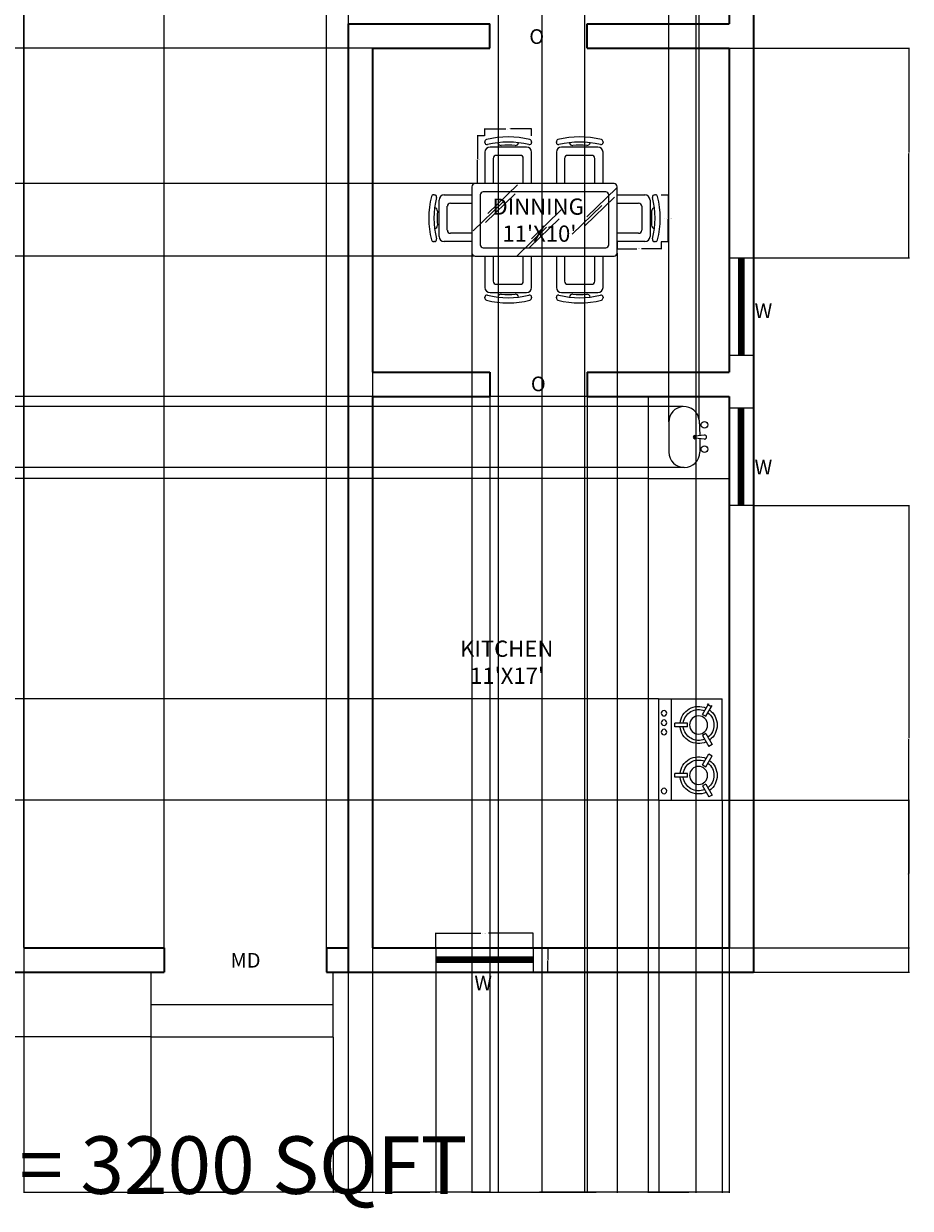
# Model space of a CAD drawing. Units: inches. Extents: x 318 to 927, y -1130 to 13.
# Tile 7 of 17: x 599 to 927, y -1130 to -692. Entities that reach past the tile are written whole.
import ezdxf

# ---------------------------------------------------------------- set-up
doc = ezdxf.new("R2010")
doc.units = ezdxf.units.IN
doc.header["$MEASUREMENT"] = 0
for name, color, linetype, lineweight in [('A-ANNO-DIMS', 1, 'Continuous', 18), ('A-ANNO-IDEN', 1, 'Continuous', 13), ('A-ANNO-TEXT', 8, 'Continuous', 25), ('A-AREA-IDEN', 8, 'Continuous', 18), ('A-EQPM', 50, 'Continuous', 18), ('A-FLOR-CASE', 50, 'Continuous', 18), ('A-FLOR-FIXT', 7, 'Continuous', 18), ('A-FLOR-STRS', 1, 'Continuous', 18), ('A-GLAZ-PATT', 5, 'Continuous', 9), ('wall', 1, 'Continuous', 35), ('win', 5, 'Continuous', 18)]:
    doc.layers.add(name, color=color, linetype=linetype, lineweight=lineweight)
doc.layers.add('furniture', color=50, linetype='Continuous', lineweight=13, transparency=0.8)
doc.styles.get("Standard").update_dxf_attribs({"font": 'arial.ttf'})
doc.dimstyles.get("Standard").update_dxf_attribs({"dimtxt": 0.18, "dimasz": 0.18, "dimexe": 0.18, "dimexo": 0.0625, "dimgap": 0.09, "dimtad": 0, "dimtih": 1, "dimtoh": 1, "dimdec": 1, "dimzin": 0, "dimdsep": 46, "dimlunit": 4, "dimtxsty": 'Standard', "dimcen": 0.09, "dimadec": 0, "dimazin": 0, "dimtfac": 1, "dimtdec": 1, "dimtofl": 0, "dimtmove": 0, "dimatfit": 3, "dimfxl": 1, "dimtolj": 1, "dimtzin": 0, "dimarcsym": 0})

# ---------------------------------------------------------------- blocks, each defined once
blk = doc.blocks.new('WIN-36IN')
for p, q in [((0, 36), (9, 36)), ((3.5, 36), (3.5, 0)), ((5.5, 36), (5.5, 0)), ((0, 0), (9, 0))]:
    blk.add_line(p, q)
blk = doc.blocks.new('CHAIR-DINING-SIDE')
for p, q in [((15.35, 13.5), (1.92, 13.5)), ((4.8, 15.13), (4.8, 15.25)), ((12.47, 15.13), (12.47, 15.25)), ((0, 11.76), (0, 11.36)), ((0, 11.58), (0, 0)), ((3.07, 9.28), (3.07, 0)), ((13.05, 10.43), (4.22, 10.43)), ((14.2, 0), (14.2, 9.28)), ((17.27, 11.36), (17.27, 11.76)), ((17.27, 0), (17.27, 11.58))]:
    blk.add_line(p, q)
for centre, radius, start, end in [((0.77, 15.54), 0.768, 104.147, 185.9216), ((-1.14, 15.34), 1.15, 354.0784, 5.9216), ((0.77, 15.15), 0.768, 174.0784, 284.3214), ((1.92, 11.58), 1.92, 90, 180), ((8.63, -15.67), 32.96, 75.853, 104.147), ((8.63, -15.67), 31.04, 75.6786, 104.3214), ((5.95, 15.25), 1.15, 186.0281, 274.9654), ((8.63, -15.67), 29.89, 85.0346, 94.9654), ((11.32, 15.25), 1.15, 265.0346, 353.9719), ((15.35, 11.58), 1.92, 0, 90), ((16.5, 15.15), 0.768, 255.6786, 5.9216), ((16.5, 15.54), 0.768, 354.0784, 75.853), ((18.41, 15.34), 1.15, 174.0784, 185.9216), ((4.22, 9.28), 1.15, 90, 180), ((13.05, 9.28), 1.15, 0, 90)]:
    blk.add_arc(centre, radius, start, end)
blk = doc.blocks.new('CHAIR-DINING-END')
for p, q in [((3.78, 1.92), (3.78, 15.35)), ((5.53, 17.27), (5.92, 17.27)), ((5.7, 17.27), (15.95, 17.27)), ((8.01, 14.2), (15.95, 14.2)), ((2.16, 12.47), (2.04, 12.47)), ((6.85, 4.22), (6.85, 13.05)), ((2.16, 4.8), (2.04, 4.8)), ((5.92, 0), (5.53, 0)), ((15.95, 0), (5.7, 0)), ((15.95, 3.07), (8.01, 3.07))]:
    blk.add_line(p, q)
for centre, radius, start, end in [((32.95, 8.63), 32.96, 165.853, 194.147), ((1.74, 16.5), 0.768, 84.0784, 165.853), ((1.94, 18.41), 1.15, 264.0784, 275.9216), ((32.95, 8.63), 31.04, 165.6786, 194.3214), ((2.14, 16.5), 0.768, 345.6786, 95.9216), ((5.7, 15.35), 1.92, 90, 180), ((8.01, 13.05), 1.15, 90, 180), ((2.04, 11.32), 1.15, 355.0346, 83.9719), ((32.95, 8.63), 29.89, 175.0346, 184.9654), ((2.04, 5.95), 1.15, 276.0281, 4.9654), ((1.74, 0.77), 0.768, 194.147, 275.9216), ((1.94, -1.14), 1.15, 84.0784, 95.9216), ((2.14, 0.77), 0.768, 264.0784, 14.3214), ((5.7, 1.92), 1.92, 180, 270), ((8.01, 4.22), 1.15, 180, 270)]:
    blk.add_arc(centre, radius, start, end)
blk = doc.blocks.new('*D11')
at = {"layer": 'A-ANNO-DIMS', "color": 0, "lineweight": -2, "transparency": 16777216}
for p, q in [((751.43, -1033.85), (751.43, -1028.33)), ((751.61, -1028.51), (768.05, -1028.51)), ((787.25, -1028.51), (770.81, -1028.51)), ((787.43, -1033.85), (787.43, -1028.33))]:
    blk.add_line(p, q, dxfattribs=at)
at = {"layer": 'A-ANNO-DIMS', "color": 0, "transparency": 16777216}
for points in [[(751.61, -1028.48), (751.61, -1028.54), (751.43, -1028.51)], [(787.25, -1028.48), (787.25, -1028.54), (787.43, -1028.51)]]:
    blk.add_solid(points, dxfattribs=at)
at = {"layer": 'Defpoints', "color": 0, "transparency": 16777216}
for p in [(787.43, -1028.51), (751.43, -1033.91), (787.43, -1033.91)]:
    blk.add_point(p, dxfattribs=at)
at = {"layer": 'A-ANNO-DIMS', "color": 0, "transparency": 16777216, "insert": (769.43, -1028.51), "char_height": 0.18, "attachment_point": 5}
blk.add_mtext('\\A1;WINDOW W 3\'-0" TYP.', dxfattribs=at)
blk = doc.blocks.new('*D12')
at = {"layer": 'A-ANNO-DIMS', "color": 0, "lineweight": -2, "transparency": 16777216}
for p, q in [((787.49, -1033.91), (793.01, -1033.91)), ((792.83, -1034.09), (792.83, -1038.23)), ((792.83, -1042.73), (792.83, -1038.59)), ((787.49, -1042.91), (793.01, -1042.91))]:
    blk.add_line(p, q, dxfattribs=at)
at = {"layer": 'A-ANNO-DIMS', "color": 0, "transparency": 16777216}
for points in [[(792.8, -1034.09), (792.86, -1034.09), (792.83, -1033.91)], [(792.8, -1042.73), (792.86, -1042.73), (792.83, -1042.91)]]:
    blk.add_solid(points, dxfattribs=at)
at = {"layer": 'Defpoints', "color": 0, "transparency": 16777216}
for p in [(787.43, -1033.91), (787.43, -1042.91), (792.83, -1042.91)]:
    blk.add_point(p, dxfattribs=at)
at = {"layer": 'A-ANNO-DIMS', "color": 0, "transparency": 16777216, "insert": (792.83, -1038.41), "char_height": 0.18, "attachment_point": 5}
blk.add_mtext('\\A1;0\'-9" TYP.', dxfattribs=at)
blk = doc.blocks.new('*D15')
at = {"layer": 'A-ANNO-DIMS', "color": 0, "lineweight": -2, "transparency": 16777216}
for p, q in [((769.42, -733.46), (766.66, -733.46)), ((766.84, -733.64), (766.84, -742.09)), ((766.84, -750.9), (766.84, -742.45)), ((769.42, -751.08), (766.66, -751.08))]:
    blk.add_line(p, q, dxfattribs=at)
at = {"layer": 'A-ANNO-DIMS', "color": 0, "transparency": 16777216}
for points in [[(766.81, -733.64), (766.87, -733.64), (766.84, -733.46)], [(766.81, -750.9), (766.87, -750.9), (766.84, -751.08)]]:
    blk.add_solid(points, dxfattribs=at)
at = {"layer": 'Defpoints', "color": 0, "transparency": 16777216}
for p in [(766.84, -733.46), (769.48, -733.46), (769.48, -751.08)]:
    blk.add_point(p, dxfattribs=at)
at = {"layer": 'A-ANNO-DIMS', "color": 0, "transparency": 16777216, "insert": (766.84, -742.27), "char_height": 0.18, "attachment_point": 5}
blk.add_mtext('\\A1;SIDE CHAIR 1\'-5 1/2" TYP.', dxfattribs=at)
blk = doc.blocks.new('*D16')
at = {"layer": 'A-ANNO-DIMS', "color": 0, "lineweight": -2, "transparency": 16777216}
for p, q in [((769.48, -733.4), (769.48, -730.64)), ((769.66, -730.82), (777.31, -730.82)), ((786.64, -730.82), (778.99, -730.82)), ((786.82, -733.4), (786.82, -730.64))]:
    blk.add_line(p, q, dxfattribs=at)
at = {"layer": 'A-ANNO-DIMS', "color": 0, "transparency": 16777216}
for points in [[(769.66, -730.79), (769.66, -730.85), (769.48, -730.82)], [(786.64, -730.79), (786.64, -730.85), (786.82, -730.82)]]:
    blk.add_solid(points, dxfattribs=at)
at = {"layer": 'Defpoints', "color": 0, "transparency": 16777216}
for p in [(786.82, -730.82), (769.48, -733.46), (786.82, -733.46)]:
    blk.add_point(p, dxfattribs=at)
at = {"layer": 'A-ANNO-DIMS', "color": 0, "transparency": 16777216, "insert": (778.15, -730.82), "char_height": 0.18, "attachment_point": 5}
blk.add_mtext('\\A1;1\'-5 1/2" TYP.', dxfattribs=at)
blk = doc.blocks.new('*D23')
at = {"layer": 'A-ANNO-DIMS', "color": 0, "lineweight": -2, "transparency": 16777216}
for p, q in [((834.8, -755.24), (837.52, -755.24)), ((837.34, -755.42), (837.34, -763.72)), ((837.34, -772.4), (837.34, -764.09)), ((834.8, -772.58), (837.52, -772.58))]:
    blk.add_line(p, q, dxfattribs=at)
at = {"layer": 'A-ANNO-DIMS', "color": 0, "transparency": 16777216}
for points in [[(837.31, -755.42), (837.37, -755.42), (837.34, -755.24)], [(837.31, -772.4), (837.37, -772.4), (837.34, -772.58)]]:
    blk.add_solid(points, dxfattribs=at)
at = {"layer": 'Defpoints', "color": 0, "transparency": 16777216}
for p in [(834.74, -755.24), (834.74, -772.58), (837.34, -772.58)]:
    blk.add_point(p, dxfattribs=at)
at = {"layer": 'A-ANNO-DIMS', "color": 0, "transparency": 16777216, "insert": (837.34, -763.91), "char_height": 0.18, "attachment_point": 5}
blk.add_mtext('\\A1;END CHAIR 1\'-5 1/2" TYP.', dxfattribs=at)
blk = doc.blocks.new('*D24')
at = {"layer": 'A-ANNO-DIMS', "color": 0, "lineweight": -2, "transparency": 16777216}
for p, q in [((818.46, -772.64), (818.46, -775.36)), ((818.64, -775.18), (825.76, -775.18)), ((834.56, -775.18), (827.44, -775.18)), ((834.74, -772.64), (834.74, -775.36))]:
    blk.add_line(p, q, dxfattribs=at)
at = {"layer": 'A-ANNO-DIMS', "color": 0, "transparency": 16777216}
for points in [[(818.64, -775.15), (818.64, -775.21), (818.46, -775.18)], [(834.56, -775.15), (834.56, -775.21), (834.74, -775.18)]]:
    blk.add_solid(points, dxfattribs=at)
at = {"layer": 'Defpoints', "color": 0, "transparency": 16777216}
for p in [(818.46, -772.58), (818.46, -775.18), (834.74, -772.58)]:
    blk.add_point(p, dxfattribs=at)
at = {"layer": 'A-ANNO-DIMS', "color": 0, "transparency": 16777216, "insert": (826.6, -775.18), "char_height": 0.18, "attachment_point": 5}
blk.add_mtext('\\A1;1\'-4 1/2" TYP.', dxfattribs=at)
blk = doc.blocks.new('*D25')
at = {"layer": 'A-ANNO-DIMS', "color": 0, "lineweight": -2, "transparency": 16777216}
for p, q in [((645.95, -1066.98), (645.95, -1124.59)), ((713.42, -1066.98), (713.42, -1124.59)), ((646.13, -1124.41), (679.15, -1124.41)), ((713.24, -1124.41), (680.22, -1124.41))]:
    blk.add_line(p, q, dxfattribs=at)
at = {"layer": 'A-ANNO-DIMS', "color": 0, "transparency": 16777216}
for points in [[(646.13, -1124.38), (646.13, -1124.44), (645.95, -1124.41)], [(713.24, -1124.38), (713.24, -1124.44), (713.42, -1124.41)]]:
    blk.add_solid(points, dxfattribs=at)
at = {"layer": 'Defpoints', "color": 0, "transparency": 16777216}
for p in [(645.95, -1066.91), (713.42, -1066.91), (713.42, -1124.41)]:
    blk.add_point(p, dxfattribs=at)
at = {"layer": 'A-ANNO-DIMS', "color": 0, "transparency": 16777216, "insert": (679.68, -1124.41), "char_height": 0.18, "attachment_point": 5}
blk.add_mtext('\\A1;5\'-7 1/2"', dxfattribs=at)
blk = doc.blocks.new('*D26')
at = {"layer": 'A-ANNO-DIMS', "color": 0, "lineweight": -2, "transparency": 16777216}
for p, q in [((645.89, -1042.91), (331.21, -1042.91)), ((331.39, -1043.09), (331.39, -1054.73)), ((331.39, -1066.73), (331.39, -1055.09)), ((645.89, -1066.91), (331.21, -1066.91))]:
    blk.add_line(p, q, dxfattribs=at)
at = {"layer": 'A-ANNO-DIMS', "color": 0, "transparency": 16777216}
for points in [[(331.36, -1043.09), (331.42, -1043.09), (331.39, -1042.91)], [(331.36, -1066.73), (331.42, -1066.73), (331.39, -1066.91)]]:
    blk.add_solid(points, dxfattribs=at)
at = {"layer": 'Defpoints', "color": 0, "transparency": 16777216}
for p in [(645.95, -1042.91), (331.39, -1066.91), (645.95, -1066.91)]:
    blk.add_point(p, dxfattribs=at)
at = {"layer": 'A-ANNO-DIMS', "color": 0, "transparency": 16777216, "insert": (331.39, -1054.91), "char_height": 0.18, "attachment_point": 5}
blk.add_mtext('\\A1;2\'-0"', dxfattribs=at)
blk = doc.blocks.new('*D27')
at = {"layer": 'A-ANNO-DIMS', "color": 0, "lineweight": -2, "transparency": 16777216}
for p, q in [((598.89, -309.98), (598.89, -1124.59)), ((718.89, -309.98), (718.89, -1124.59)), ((599.07, -1124.41), (658.5, -1124.41)), ((718.71, -1124.41), (659.28, -1124.41))]:
    blk.add_line(p, q, dxfattribs=at)
at = {"layer": 'A-ANNO-DIMS', "color": 0, "transparency": 16777216}
for points in [[(599.07, -1124.38), (599.07, -1124.44), (598.89, -1124.41)], [(718.71, -1124.38), (718.71, -1124.44), (718.89, -1124.41)]]:
    blk.add_solid(points, dxfattribs=at)
at = {"layer": 'Defpoints', "color": 0, "transparency": 16777216}
for p in [(598.89, -309.91), (718.89, -309.91), (718.89, -1124.41)]:
    blk.add_point(p, dxfattribs=at)
at = {"layer": 'A-ANNO-DIMS', "color": 0, "transparency": 16777216, "insert": (658.89, -1124.41), "char_height": 0.18, "attachment_point": 5}
blk.add_mtext('\\A1;10\'-0"', dxfattribs=at)
blk = doc.blocks.new('*D28')
at = {"layer": 'A-ANNO-DIMS', "color": 0, "lineweight": -2, "transparency": 16777216}
for p, q in [((650.89, -1033.85), (650.89, -25.23)), ((651.07, -25.41), (680.57, -25.41)), ((710.71, -25.41), (681.22, -25.41)), ((710.89, -1033.85), (710.89, -25.23))]:
    blk.add_line(p, q, dxfattribs=at)
at = {"layer": 'A-ANNO-DIMS', "color": 0, "transparency": 16777216}
for points in [[(651.07, -25.38), (651.07, -25.44), (650.89, -25.41)], [(710.71, -25.38), (710.71, -25.44), (710.89, -25.41)]]:
    blk.add_solid(points, dxfattribs=at)
at = {"layer": 'Defpoints', "color": 0, "transparency": 16777216}
for p in [(710.89, -25.41), (650.89, -1033.91), (710.89, -1033.91)]:
    blk.add_point(p, dxfattribs=at)
at = {"layer": 'A-ANNO-DIMS', "color": 0, "transparency": 16777216, "insert": (680.89, -25.41), "char_height": 0.18, "attachment_point": 5}
blk.add_mtext('\\A1;5\'-0"', dxfattribs=at)
blk = doc.blocks.new('*D29')
at = {"layer": 'A-ANNO-DIMS', "color": 0, "lineweight": -2, "transparency": 16777216}
for p, q in [((598.89, -1033.85), (598.89, -25.23)), ((599.07, -25.41), (624.56, -25.41)), ((650.71, -25.41), (625.23, -25.41)), ((650.89, -1033.85), (650.89, -25.23))]:
    blk.add_line(p, q, dxfattribs=at)
at = {"layer": 'A-ANNO-DIMS', "color": 0, "transparency": 16777216}
for points in [[(599.07, -25.38), (599.07, -25.44), (598.89, -25.41)], [(650.71, -25.38), (650.71, -25.44), (650.89, -25.41)]]:
    blk.add_solid(points, dxfattribs=at)
at = {"layer": 'Defpoints', "color": 0, "transparency": 16777216}
for p in [(650.89, -25.41), (598.89, -1033.91), (650.89, -1033.91)]:
    blk.add_point(p, dxfattribs=at)
at = {"layer": 'A-ANNO-DIMS', "color": 0, "transparency": 16777216, "insert": (624.89, -25.41), "char_height": 0.18, "attachment_point": 5}
blk.add_mtext('\\A1;4\'-4"', dxfattribs=at)
blk = doc.blocks.new('*D39')
at = {"layer": 'A-ANNO-DIMS', "color": 0, "lineweight": -2, "transparency": 16777216}
for p, q in [((847.56, -595.87), (847.56, -1124.59)), ((774.46, -617.18), (774.46, -1124.59)), ((774.64, -1124.41), (810.68, -1124.41)), ((847.38, -1124.41), (811.34, -1124.41))]:
    blk.add_line(p, q, dxfattribs=at)
at = {"layer": 'A-ANNO-DIMS', "color": 0, "transparency": 16777216}
for points in [[(774.64, -1124.38), (774.64, -1124.44), (774.46, -1124.41)], [(847.38, -1124.38), (847.38, -1124.44), (847.56, -1124.41)]]:
    blk.add_solid(points, dxfattribs=at)
at = {"layer": 'Defpoints', "color": 0, "transparency": 16777216}
for p in [(847.56, -595.81), (774.46, -617.11), (847.56, -1124.41)]:
    blk.add_point(p, dxfattribs=at)
at = {"layer": 'A-ANNO-DIMS', "color": 0, "transparency": 16777216, "insert": (811.01, -1124.41), "char_height": 0.18, "attachment_point": 5}
blk.add_mtext('\\A1;6\'-1"', dxfattribs=at)
blk = doc.blocks.new('*D40')
at = {"layer": 'A-ANNO-DIMS', "color": 0, "lineweight": -2, "transparency": 16777216}
for p, q in [((790.65, -580.99), (790.65, -1124.59)), ((806.39, -580.99), (806.39, -1124.59)), ((790.83, -1124.41), (797.99, -1124.41)), ((806.21, -1124.41), (799.05, -1124.41))]:
    blk.add_line(p, q, dxfattribs=at)
at = {"layer": 'A-ANNO-DIMS', "color": 0, "transparency": 16777216}
for points in [[(790.83, -1124.38), (790.83, -1124.44), (790.65, -1124.41)], [(806.21, -1124.38), (806.21, -1124.44), (806.39, -1124.41)]]:
    blk.add_solid(points, dxfattribs=at)
at = {"layer": 'Defpoints', "color": 0, "transparency": 16777216}
for p in [(790.65, -580.93), (806.39, -580.93), (806.39, -1124.41)]:
    blk.add_point(p, dxfattribs=at)
at = {"layer": 'A-ANNO-DIMS', "color": 0, "transparency": 16777216, "insert": (798.52, -1124.41), "char_height": 0.18, "attachment_point": 5}
blk.add_mtext('\\A1;1\'-3 1/2"', dxfattribs=at)
blk = doc.blocks.new('*D45')
at = {"layer": 'A-ANNO-DIMS', "color": 0, "lineweight": -2, "transparency": 16777216}
for p, q in [((829.89, -1033.98), (829.89, -1124.59)), ((859.89, -1033.98), (859.89, -1124.59)), ((830.07, -1124.41), (844.56, -1124.41)), ((859.71, -1124.41), (845.23, -1124.41))]:
    blk.add_line(p, q, dxfattribs=at)
at = {"layer": 'A-ANNO-DIMS', "color": 0, "transparency": 16777216}
for points in [[(830.07, -1124.38), (830.07, -1124.44), (829.89, -1124.41)], [(859.71, -1124.38), (859.71, -1124.44), (859.89, -1124.41)]]:
    blk.add_solid(points, dxfattribs=at)
at = {"layer": 'Defpoints', "color": 0, "transparency": 16777216}
for p in [(829.89, -1033.91), (859.89, -1033.91), (859.89, -1124.41)]:
    blk.add_point(p, dxfattribs=at)
at = {"layer": 'A-ANNO-DIMS', "color": 0, "transparency": 16777216, "insert": (844.89, -1124.41), "char_height": 0.18, "attachment_point": 5}
blk.add_mtext('\\A1;2\'-6"', dxfattribs=at)
blk = doc.blocks.new('*D46')
at = {"layer": 'A-ANNO-DIMS', "color": 0, "lineweight": -2, "transparency": 16777216}
for p, q in [((771.39, -829.98), (771.39, -1124.59)), ((807.39, -829.98), (807.39, -1124.59)), ((771.57, -1124.41), (789.07, -1124.41)), ((807.21, -1124.41), (789.72, -1124.41))]:
    blk.add_line(p, q, dxfattribs=at)
at = {"layer": 'A-ANNO-DIMS', "color": 0, "transparency": 16777216}
for points in [[(771.57, -1124.38), (771.57, -1124.44), (771.39, -1124.41)], [(807.21, -1124.38), (807.21, -1124.44), (807.39, -1124.41)]]:
    blk.add_solid(points, dxfattribs=at)
at = {"layer": 'Defpoints', "color": 0, "transparency": 16777216}
for p in [(771.39, -829.91), (807.39, -829.91), (807.39, -1124.41)]:
    blk.add_point(p, dxfattribs=at)
at = {"layer": 'A-ANNO-DIMS', "color": 0, "transparency": 16777216, "insert": (789.39, -1124.41), "char_height": 0.18, "attachment_point": 5}
blk.add_mtext('\\A1;3\'-0"', dxfattribs=at)
blk = doc.blocks.new('*D47')
at = {"layer": 'A-ANNO-DIMS', "color": 0, "lineweight": -2, "transparency": 16777216}
for p, q in [((727.89, -829.98), (727.89, -1124.59)), ((771.39, -829.98), (771.39, -1124.59)), ((728.07, -1124.41), (749.11, -1124.41)), ((771.21, -1124.41), (750.18, -1124.41))]:
    blk.add_line(p, q, dxfattribs=at)
at = {"layer": 'A-ANNO-DIMS', "color": 0, "transparency": 16777216}
for points in [[(728.07, -1124.38), (728.07, -1124.44), (727.89, -1124.41)], [(771.21, -1124.38), (771.21, -1124.44), (771.39, -1124.41)]]:
    blk.add_solid(points, dxfattribs=at)
at = {"layer": 'Defpoints', "color": 0, "transparency": 16777216}
for p in [(727.89, -829.91), (771.39, -829.91), (771.39, -1124.41)]:
    blk.add_point(p, dxfattribs=at)
at = {"layer": 'A-ANNO-DIMS', "color": 0, "transparency": 16777216, "insert": (749.64, -1124.41), "char_height": 0.18, "attachment_point": 5}
blk.add_mtext('\\A1;3\'-7 1/2"', dxfattribs=at)
blk = doc.blocks.new('*D48')
at = {"layer": 'A-ANNO-DIMS', "color": 0, "lineweight": -2, "transparency": 16777216}
for p, q in [((764.73, -776.85), (764.73, -1124.59)), ((818.46, -776.85), (818.46, -1124.59)), ((764.91, -1124.41), (791.05, -1124.41)), ((818.28, -1124.41), (792.14, -1124.41))]:
    blk.add_line(p, q, dxfattribs=at)
at = {"layer": 'A-ANNO-DIMS', "color": 0, "transparency": 16777216}
for points in [[(764.91, -1124.38), (764.91, -1124.44), (764.73, -1124.41)], [(818.28, -1124.38), (818.28, -1124.44), (818.46, -1124.41)]]:
    blk.add_solid(points, dxfattribs=at)
at = {"layer": 'Defpoints', "color": 0, "transparency": 16777216}
for p in [(764.73, -776.79), (818.46, -776.79), (818.46, -1124.41)]:
    blk.add_point(p, dxfattribs=at)
at = {"layer": 'A-ANNO-DIMS', "color": 0, "transparency": 16777216, "insert": (791.6, -1124.41), "char_height": 0.18, "attachment_point": 5}
blk.add_mtext('\\A1;4\'-5 1/2"', dxfattribs=at)
blk = doc.blocks.new('*D49')
at = {"layer": 'A-ANNO-DIMS', "color": 0, "lineweight": -2, "transparency": 16777216}
for p, q in [((765.82, -751.08), (331.21, -751.08)), ((331.39, -751.26), (331.39, -764.33)), ((331.39, -777.76), (331.39, -764.69)), ((765.82, -777.94), (331.21, -777.94))]:
    blk.add_line(p, q, dxfattribs=at)
at = {"layer": 'A-ANNO-DIMS', "color": 0, "transparency": 16777216}
for points in [[(331.36, -751.26), (331.42, -751.26), (331.39, -751.08)], [(331.36, -777.76), (331.42, -777.76), (331.39, -777.94)]]:
    blk.add_solid(points, dxfattribs=at)
at = {"layer": 'Defpoints', "color": 0, "transparency": 16777216}
for p in [(765.88, -751.08), (331.39, -777.94), (765.88, -777.94)]:
    blk.add_point(p, dxfattribs=at)
at = {"layer": 'A-ANNO-DIMS', "color": 0, "transparency": 16777216, "insert": (331.39, -764.51), "char_height": 0.18, "attachment_point": 5}
blk.add_mtext('\\A1;2\'-3"', dxfattribs=at)
blk = doc.blocks.new('*D50')
at = {"layer": 'A-ANNO-DIMS', "color": 0, "lineweight": -2, "transparency": 16777216}
for p, q in [((764.73, -776.85), (764.73, -1124.59)), ((727.89, -820.98), (727.89, -1124.59)), ((728.07, -1124.41), (745.98, -1124.41)), ((764.55, -1124.41), (746.64, -1124.41))]:
    blk.add_line(p, q, dxfattribs=at)
at = {"layer": 'A-ANNO-DIMS', "color": 0, "transparency": 16777216}
for points in [[(728.07, -1124.38), (728.07, -1124.44), (727.89, -1124.41)], [(764.55, -1124.38), (764.55, -1124.44), (764.73, -1124.41)]]:
    blk.add_solid(points, dxfattribs=at)
at = {"layer": 'Defpoints', "color": 0, "transparency": 16777216}
for p in [(764.73, -776.79), (727.89, -820.91), (764.73, -1124.41)]:
    blk.add_point(p, dxfattribs=at)
at = {"layer": 'A-ANNO-DIMS', "color": 0, "transparency": 16777216, "insert": (746.31, -1124.41), "char_height": 0.18, "attachment_point": 5}
blk.add_mtext('\\A1;3\'-1"', dxfattribs=at)
blk = doc.blocks.new('*D51')
at = {"layer": 'A-ANNO-DIMS', "color": 0, "lineweight": -2, "transparency": 16777216}
for p, q in [((771.33, -700.91), (331.21, -700.91)), ((331.39, -701.09), (331.39, -725.82)), ((331.39, -750.9), (331.39, -726.18)), ((765.82, -751.08), (331.21, -751.08))]:
    blk.add_line(p, q, dxfattribs=at)
at = {"layer": 'A-ANNO-DIMS', "color": 0, "transparency": 16777216}
for points in [[(331.36, -701.09), (331.42, -701.09), (331.39, -700.91)], [(331.36, -750.9), (331.42, -750.9), (331.39, -751.08)]]:
    blk.add_solid(points, dxfattribs=at)
at = {"layer": 'Defpoints', "color": 0, "transparency": 16777216}
for p in [(771.39, -700.91), (331.39, -751.08), (765.88, -751.08)]:
    blk.add_point(p, dxfattribs=at)
at = {"layer": 'A-ANNO-DIMS', "color": 0, "transparency": 16777216, "insert": (331.39, -726), "char_height": 0.18, "attachment_point": 5}
blk.add_mtext('\\A1;4\'-2"', dxfattribs=at)
blk = doc.blocks.new('*D52')
at = {"layer": 'A-ANNO-DIMS', "color": 0, "lineweight": -2, "transparency": 16777216}
for p, q in [((829.83, -829.91), (331.21, -829.91)), ((331.39, -830.09), (331.39, -844.92)), ((331.39, -860.11), (331.39, -845.29)), ((829.83, -860.29), (331.21, -860.29))]:
    blk.add_line(p, q, dxfattribs=at)
at = {"layer": 'A-ANNO-DIMS', "color": 0, "transparency": 16777216}
for points in [[(331.36, -830.09), (331.42, -830.09), (331.39, -829.91)], [(331.36, -860.11), (331.42, -860.11), (331.39, -860.29)]]:
    blk.add_solid(points, dxfattribs=at)
at = {"layer": 'Defpoints', "color": 0, "transparency": 16777216}
for p in [(829.89, -829.91), (331.39, -860.29), (829.89, -860.29)]:
    blk.add_point(p, dxfattribs=at)
at = {"layer": 'A-ANNO-DIMS', "color": 0, "transparency": 16777216, "insert": (331.39, -845.1), "char_height": 0.18, "attachment_point": 5}
blk.add_mtext('\\A1;2\'-6 1/2"', dxfattribs=at)
blk = doc.blocks.new('*D53')
at = {"layer": 'A-ANNO-DIMS', "color": 0, "lineweight": -2, "transparency": 16777216}
for p, q in [((837.57, -839.31), (837.57, -25.23)), ((837.75, -25.41), (842.6, -25.41)), ((848.66, -25.41), (843.82, -25.41)), ((848.84, -838.59), (848.84, -25.23))]:
    blk.add_line(p, q, dxfattribs=at)
at = {"layer": 'A-ANNO-DIMS', "color": 0, "transparency": 16777216}
for points in [[(837.75, -25.38), (837.75, -25.44), (837.57, -25.41)], [(848.66, -25.38), (848.66, -25.44), (848.84, -25.41)]]:
    blk.add_solid(points, dxfattribs=at)
at = {"layer": 'Defpoints', "color": 0, "transparency": 16777216}
for p in [(848.84, -25.41), (837.57, -839.37), (848.84, -838.66)]:
    blk.add_point(p, dxfattribs=at)
at = {"layer": 'A-ANNO-DIMS', "color": 0, "transparency": 16777216, "insert": (843.21, -25.41), "char_height": 0.18, "attachment_point": 5}
blk.add_mtext('\\A1;0\'-11 1/2"', dxfattribs=at)
blk = doc.blocks.new('*D54')
at = {"layer": 'A-ANNO-DIMS', "color": 0, "lineweight": -2, "transparency": 16777216}
for p, q in [((842.8, -833.64), (331.21, -833.64)), ((331.39, -833.82), (331.39, -844.73)), ((331.39, -856), (331.39, -845.09)), ((843.25, -856.18), (331.21, -856.18))]:
    blk.add_line(p, q, dxfattribs=at)
at = {"layer": 'A-ANNO-DIMS', "color": 0, "transparency": 16777216}
for points in [[(331.36, -833.82), (331.42, -833.82), (331.39, -833.64)], [(331.36, -856), (331.42, -856), (331.39, -856.18)]]:
    blk.add_solid(points, dxfattribs=at)
at = {"layer": 'Defpoints', "color": 0, "transparency": 16777216}
for p in [(842.87, -833.64), (331.39, -856.18), (843.31, -856.18)]:
    blk.add_point(p, dxfattribs=at)
at = {"layer": 'A-ANNO-DIMS', "color": 0, "transparency": 16777216, "insert": (331.39, -844.91), "char_height": 0.18, "attachment_point": 5}
blk.add_mtext('\\A1;1\'-10 1/2"', dxfattribs=at)
blk = doc.blocks.new('*D55')
at = {"layer": 'A-ANNO-DIMS', "color": 0, "lineweight": -2, "transparency": 16777216}
for p, q in [((833.82, -941.75), (331.21, -941.75)), ((331.39, -941.93), (331.39, -960.35)), ((331.39, -979.13), (331.39, -960.71)), ((833.82, -979.31), (331.21, -979.31))]:
    blk.add_line(p, q, dxfattribs=at)
at = {"layer": 'A-ANNO-DIMS', "color": 0, "transparency": 16777216}
for points in [[(331.36, -941.93), (331.42, -941.93), (331.39, -941.75)], [(331.36, -979.13), (331.42, -979.13), (331.39, -979.31)]]:
    blk.add_solid(points, dxfattribs=at)
at = {"layer": 'Defpoints', "color": 0, "transparency": 16777216}
for p in [(833.89, -941.75), (331.39, -979.31), (833.89, -979.31)]:
    blk.add_point(p, dxfattribs=at)
at = {"layer": 'A-ANNO-DIMS', "color": 0, "transparency": 16777216, "insert": (331.39, -960.53), "char_height": 0.18, "attachment_point": 5}
blk.add_mtext('\\A1;3\'-1 1/2"', dxfattribs=at)
blk = doc.blocks.new('*D56')
at = {"layer": 'A-ANNO-DIMS', "color": 0, "lineweight": -2, "transparency": 16777216}
for p, q in [((833.89, -979.37), (833.89, -1124.59)), ((857.36, -979.37), (857.36, -1124.59)), ((834.07, -1124.41), (845.02, -1124.41)), ((857.18, -1124.41), (846.22, -1124.41))]:
    blk.add_line(p, q, dxfattribs=at)
at = {"layer": 'A-ANNO-DIMS', "color": 0, "transparency": 16777216}
for points in [[(834.07, -1124.38), (834.07, -1124.44), (833.89, -1124.41)], [(857.18, -1124.38), (857.18, -1124.44), (857.36, -1124.41)]]:
    blk.add_solid(points, dxfattribs=at)
at = {"layer": 'Defpoints', "color": 0, "transparency": 16777216}
for p in [(833.89, -979.31), (857.36, -979.31), (857.36, -1124.41)]:
    blk.add_point(p, dxfattribs=at)
at = {"layer": 'A-ANNO-DIMS', "color": 0, "transparency": 16777216, "insert": (845.62, -1124.41), "char_height": 0.18, "attachment_point": 5}
blk.add_mtext('\\A1;1\'-11 1/2"', dxfattribs=at)
blk = doc.blocks.new('*D57')
at = {"layer": 'A-ANNO-DIMS', "color": 0, "lineweight": -2, "transparency": 16777216}
for p, q in [((857.42, -979.31), (926.57, -979.31)), ((926.39, -979.49), (926.39, -1006.43)), ((926.39, -1033.73), (926.39, -1006.79)), ((859.96, -1033.91), (926.57, -1033.91))]:
    blk.add_line(p, q, dxfattribs=at)
at = {"layer": 'A-ANNO-DIMS', "color": 0, "transparency": 16777216}
for points in [[(926.36, -979.49), (926.42, -979.49), (926.39, -979.31)], [(926.36, -1033.73), (926.42, -1033.73), (926.39, -1033.91)]]:
    blk.add_solid(points, dxfattribs=at)
at = {"layer": 'Defpoints', "color": 0, "transparency": 16777216}
for p in [(857.36, -979.31), (859.89, -1033.91), (926.39, -1033.91)]:
    blk.add_point(p, dxfattribs=at)
at = {"layer": 'A-ANNO-DIMS', "color": 0, "transparency": 16777216, "insert": (926.39, -1006.61), "char_height": 0.18, "attachment_point": 5}
blk.add_mtext('\\A1;4\'-6 1/2"', dxfattribs=at)
blk = doc.blocks.new('*D58')
at = {"layer": 'A-ANNO-DIMS', "color": 0, "lineweight": -2, "transparency": 16777216}
for p, q in [((718.89, -1042.98), (718.89, -1124.59)), ((751.43, -1042.98), (751.43, -1124.59)), ((719.07, -1124.41), (734.62, -1124.41)), ((751.25, -1124.41), (735.7, -1124.41))]:
    blk.add_line(p, q, dxfattribs=at)
at = {"layer": 'A-ANNO-DIMS', "color": 0, "transparency": 16777216}
for points in [[(719.07, -1124.38), (719.07, -1124.44), (718.89, -1124.41)], [(751.25, -1124.38), (751.25, -1124.44), (751.43, -1124.41)]]:
    blk.add_solid(points, dxfattribs=at)
at = {"layer": 'Defpoints', "color": 0, "transparency": 16777216}
for p in [(718.89, -1042.91), (751.43, -1042.91), (751.43, -1124.41)]:
    blk.add_point(p, dxfattribs=at)
at = {"layer": 'A-ANNO-DIMS', "color": 0, "transparency": 16777216, "insert": (735.16, -1124.41), "char_height": 0.18, "attachment_point": 5}
blk.add_mtext('\\A1;2\'-8 1/2"', dxfattribs=at)
blk = doc.blocks.new('*D59')
at = {"layer": 'A-ANNO-DIMS', "color": 0, "lineweight": -2, "transparency": 16777216}
for p, q in [((868.96, -870.21), (926.57, -870.21)), ((926.39, -870.39), (926.39, -956.38)), ((926.39, -1042.73), (926.39, -956.74)), ((868.96, -1042.91), (926.57, -1042.91))]:
    blk.add_line(p, q, dxfattribs=at)
at = {"layer": 'A-ANNO-DIMS', "color": 0, "transparency": 16777216}
for points in [[(926.36, -870.39), (926.42, -870.39), (926.39, -870.21)], [(926.36, -1042.73), (926.42, -1042.73), (926.39, -1042.91)]]:
    blk.add_solid(points, dxfattribs=at)
at = {"layer": 'Defpoints', "color": 0, "transparency": 16777216}
for p in [(868.89, -870.21), (926.39, -870.21), (868.89, -1042.91)]:
    blk.add_point(p, dxfattribs=at)
at = {"layer": 'A-ANNO-DIMS', "color": 0, "transparency": 16777216, "insert": (926.39, -956.56), "char_height": 0.18, "attachment_point": 5}
blk.add_mtext('\\A1;14\'-4 1/2"', dxfattribs=at)
blk = doc.blocks.new('*D64')
at = {"layer": 'A-ANNO-DIMS', "color": 0, "lineweight": -2, "transparency": 16777216}
for p, q in [((859.96, -700.91), (926.57, -700.91)), ((926.39, -701.09), (926.39, -739.57)), ((926.39, -778.42), (926.39, -739.94)), ((859.96, -778.6), (926.57, -778.6))]:
    blk.add_line(p, q, dxfattribs=at)
at = {"layer": 'A-ANNO-DIMS', "color": 0, "transparency": 16777216}
for points in [[(926.36, -701.09), (926.42, -701.09), (926.39, -700.91)], [(926.36, -778.42), (926.42, -778.42), (926.39, -778.6)]]:
    blk.add_solid(points, dxfattribs=at)
at = {"layer": 'Defpoints', "color": 0, "transparency": 16777216}
for p in [(859.89, -700.91), (859.89, -778.6), (926.39, -778.6)]:
    blk.add_point(p, dxfattribs=at)
at = {"layer": 'A-ANNO-DIMS', "color": 0, "transparency": 16777216, "insert": (926.39, -739.75), "char_height": 0.18, "attachment_point": 5}
blk.add_mtext('\\A1;6\'-5 1/2"', dxfattribs=at)

msp = doc.modelspace()

# ---------------------------------------------------------------- hatches: boundary and pattern name
at = {"layer": 'A-GLAZ-PATT'}
h = msp.add_hatch(dxfattribs=at)
h.set_pattern_fill('ANSI31', color=256)
h.paths.add_polyline_path([(865.39, -312.52), (863.39, -312.52), (863.39, -348.52), (865.39, -348.52)])
h.paths.add_polyline_path([(865.39, -440.16), (863.39, -440.16), (863.39, -488.16), (865.39, -488.16)])
h.paths.add_polyline_path([(865.39, -635.51), (863.39, -635.51), (863.39, -683.51), (865.39, -683.51)])
h.paths.add_polyline_path([(865.39, -778.6), (863.39, -778.6), (863.39, -814.6), (865.39, -814.6)])
h.paths.add_polyline_path([(865.39, -834.21), (863.39, -834.21), (863.39, -870.21), (865.39, -870.21)])
h = msp.add_hatch(dxfattribs=at)
h.set_pattern_fill('ANSI31', color=256)
h.paths.add_polyline_path([(787.43, -1037.41), (751.43, -1037.41), (751.43, -1039.41), (787.43, -1039.41)])
h.paths.add_polyline_path([(583.67, -1037.41), (547.67, -1037.41), (547.67, -1039.41), (583.67, -1039.41)])
h.paths.add_polyline_path([(394.39, -842.15), (392.39, -842.15), (392.39, -878.15), (394.39, -878.15)])
h.paths.add_polyline_path([(394.39, -788.96), (392.39, -788.96), (392.39, -812.96), (394.39, -812.96)])

# ---------------------------------------------------------------- linework, layer by layer
at = {"layer": 'A-EQPM'}
for p, q in [((833.89, -979.31), (833.89, -941.75)), ((833.89, -941.75), (857.36, -941.75)), ((838.58, -979.31), (838.58, -941.75)), ((857.36, -979.31), (857.36, -941.75)), ((850.02, -947.55), (852.36, -943.5)), ((851.24, -948.25), (853.58, -944.2)), ((851.81, -943.69), (853.17, -944.47)), ((844.47, -950.75), (839.79, -950.75)), ((839.79, -952.16), (839.79, -950.75)), ((844.47, -952.16), (844.47, -950.75)), ((850.02, -947.55), (851.24, -948.25)), ((844.47, -952.16), (839.79, -952.16)), ((851.24, -954.67), (850.02, -955.37)), ((850.02, -955.37), (852.36, -959.42)), ((851.24, -954.67), (853.58, -958.72)), ((853.58, -958.72), (852.36, -959.42)), ((850.02, -966.21), (852.36, -962.16)), ((851.24, -966.91), (853.58, -962.86)), ((852.36, -962.16), (853.58, -962.86)), ((850.02, -966.21), (851.24, -966.91)), ((844.47, -969.41), (839.79, -969.41)), ((839.79, -970.82), (839.79, -969.41)), ((844.47, -970.82), (839.79, -970.82)), ((844.47, -970.82), (844.47, -969.41)), ((851.24, -973.33), (850.02, -974.03)), ((850.02, -974.03), (852.36, -978.08)), ((851.24, -973.33), (853.58, -977.38)), ((853.58, -977.38), (852.36, -978.08)), ((833.89, -979.31), (857.36, -979.31))]:
    msp.add_line(p, q, dxfattribs=at)
at = {"layer": 'A-EQPM', "extrusion": (0, 0, -1)}
for centre, major_axis, start_param, end_param in [((835.81, -947.1), (0.72, 0.72), 2.35619449019219, 8.639379797371777), ((848.58, -951.46), (6.88, 0), 3.2451, 5.134376), ((848.58, -951.46), (4.03, 4.03), 4.051123, 5.898002), ((848.58, -951.46), (4.03, 4.03), 6.145519, 7.992397), ((848.58, -951.46), (6.88, 0.01), -0.942584, 0.946692), ((835.81, -950.63), (0.72, 0.72), 2.35619449019219, 8.639379797371777), ((848.58, -951.46), (2.37, 2.37), 2.356194490192312, 8.639379797371898), ((835.81, -954.08), (0.72, 0.72), 2.35619449019219, 8.639379797371777), ((848.58, -951.46), (6.88, -0.01), 1.148752, 3.038029), ((848.58, -951.46), (4.03, -4.03), 0.385932, 2.23281), ((848.58, -970.12), (6.88, 0), 3.244173, 5.13345), ((848.58, -970.12), (4.03, -4.03), 2.480327, 4.327205), ((848.58, -970.12), (2.37, 2.37), 2.356194490192306, 8.639379797371893), ((848.58, -970.12), (4.03, 4.03), 6.145519, 7.992397), ((848.58, -970.12), (6.88, 0), -0.944011, 0.945266), ((848.58, -970.12), (6.88, -0.01), 1.14879, 3.038067), ((848.58, -970.12), (4.03, -4.03), 0.385932, 2.23281), ((835.81, -975.88), (0.72, 0.72), 2.35619449019219, 8.639379797371777)]:
    msp.add_ellipse(centre, major_axis=major_axis, ratio=1, start_param=start_param, end_param=end_param, dxfattribs=at)
at = {"layer": 'A-FLOR-CASE'}
for p, q in [((829.89, -829.91), (829.89, -1033.91)), ((829.89, -860.29), (859.89, -860.29))]:
    msp.add_line(p, q, dxfattribs=at)
at = {"layer": 'A-FLOR-FIXT'}
for p, q in [((837.57, -839.37), (837.57, -850.44)), ((848.84, -838.66), (849, -844.29)), ((847.26, -844.49), (850.74, -844.08)), ((847.26, -845.37), (847.26, -844.49)), ((850.74, -845.72), (847.26, -845.31)), ((849.05, -845.53), (849.05, -850.44))]:
    msp.add_line(p, q, dxfattribs=at)
for centre in [(850.74, -840.4), (850.74, -849.41)]:
    msp.add_circle(centre, 1.23, dxfattribs=at)
for centre, radius, start, end in [((843.22, -839.28), 5.65, 6.3659, 180.8792), ((847.26, -844.9), 0.615, 48.1701, 311.8299), ((850.74, -844.9), 0.82, 270, 90), ((843.31, -850.44), 5.74, 180, 0)]:
    msp.add_arc(centre, radius, start, end, dxfattribs=at)
at = {"layer": 'A-FLOR-STRS'}
for p, q in [((645.95, -1042.91), (645.95, -1066.91)), ((713.42, -1066.91), (713.42, -1042.91)), ((645.95, -1054.91), (713.42, -1054.91)), ((645.95, -1066.91), (713.42, -1066.91))]:
    msp.add_line(p, q, dxfattribs=at)
at = {"layer": 'furniture'}
for p, q in [((764.73, -752.23), (764.73, -776.79)), ((817.31, -751.08), (765.88, -751.08)), ((781.55, -751.58), (770.57, -762.21)), ((818.21, -752.76), (807.23, -763.39)), ((818.46, -776.79), (818.46, -752.23)), ((776.12, -757.98), (765.14, -768.61)), ((767.8, -755.3), (767.8, -773.72)), ((814.24, -754.15), (768.95, -754.15)), ((780.79, -754.89), (769.81, -765.52)), ((817.45, -756.07), (806.47, -766.7)), ((815.39, -773.72), (815.39, -755.3)), ((797.77, -760.86), (786.79, -771.49)), ((812.78, -759.16), (801.8, -769.79)), ((797.01, -764.17), (786.03, -774.8)), ((792.34, -767.26), (781.35, -777.89)), ((768.95, -774.87), (814.24, -774.87)), ((765.88, -777.94), (817.31, -777.94))]:
    msp.add_line(p, q, dxfattribs=at)
for centre, radius, start, end in [((765.88, -752.23), 1.15, 90, 180), ((817.36, -752.18), 1.1, 357.166, 92.834), ((768.95, -755.3), 1.15, 90, 180), ((814.24, -755.3), 1.15, 0, 90), ((768.95, -773.72), 1.15, 180, 270), ((814.24, -773.72), 1.15, 270, 0), ((765.88, -776.79), 1.15, 180, 270), ((817.31, -776.79), 1.15, 270, 0)]:
    msp.add_arc(centre, radius, start, end, dxfattribs=at)
at = {"layer": 'wall'}
for p, q in [((868.89, -82.91), (868.89, -1042.91)), ((859.89, -433.91), (859.89, -691.91)), ((718.89, -691.91), (771.39, -691.91)), ((718.89, -691.91), (771.39, -691.91)), ((718.89, -691.91), (718.89, -1042.91)), ((771.39, -700.91), (771.39, -691.91)), ((807.39, -700.91), (807.39, -691.91)), ((807.39, -691.91), (859.89, -691.91)), ((807.39, -691.91), (859.89, -691.91)), ((727.89, -700.91), (771.39, -700.91)), ((727.89, -700.91), (771.39, -700.91)), ((727.89, -700.91), (727.89, -820.91)), ((807.39, -700.91), (859.89, -700.91)), ((807.39, -700.91), (859.89, -700.91)), ((859.89, -700.91), (859.89, -820.91)), ((727.89, -820.91), (771.39, -820.91)), ((727.89, -820.91), (771.39, -820.91)), ((771.39, -820.91), (771.39, -829.91)), ((807.39, -820.91), (807.39, -829.91)), ((807.39, -820.91), (859.89, -820.91)), ((807.39, -820.91), (859.89, -820.91)), ((727.89, -829.91), (771.39, -829.91)), ((727.89, -829.91), (771.39, -829.91)), ((727.89, -829.91), (727.89, -1033.91)), ((807.39, -829.91), (859.89, -829.91)), ((807.39, -829.91), (859.89, -829.91)), ((859.89, -829.91), (859.89, -1033.91)), ((598.89, -1033.91), (650.89, -1033.91)), ((650.89, -1033.91), (650.89, -1042.91)), ((710.89, -1033.91), (710.89, -1042.91)), ((710.89, -1033.91), (718.89, -1033.91)), ((727.89, -1033.91), (859.89, -1033.91)), ((388.89, -1042.91), (650.89, -1042.91)), ((710.89, -1042.91), (868.89, -1042.91))]:
    msp.add_line(p, q, dxfattribs=at)

# ---------------------------------------------------------------- block references
at = {"layer": 'furniture'}
for name, p in [('CHAIR-DINING-SIDE', (769.52, -751.08)), ('CHAIR-DINING-SIDE', (795.97, -751.08)), ('CHAIR-DINING-END', (748.78, -772.54))]:
    msp.add_blockref(name, p, dxfattribs=at)
at = {"layer": 'furniture', "rotation": 180}
for name, p in [('CHAIR-DINING-END', (834.41, -755.27)), ('CHAIR-DINING-SIDE', (786.79, -777.94)), ('CHAIR-DINING-SIDE', (813.24, -777.94))]:
    msp.add_blockref(name, p, dxfattribs=at)
at = {"layer": 'win'}
msp.add_blockref('WIN-36IN', (859.89, -814.6), dxfattribs=at)
for p, rotation in [((868.89, -834.21), 180), ((751.43, -1033.91), 269.9999999999997)]:
    msp.add_blockref('WIN-36IN', p, dxfattribs=dict(at, rotation=rotation))

# ---------------------------------------------------------------- texts
at = {"layer": 'A-ANNO-IDEN'}
for s, height, p in [('O', 5.44, (785.95, -699.4)), ('W', 5.44, (869.32, -800.87)), ('O', 5.44, (786.54, -827.94)), ('W', 5.44, (869.32, -858.75)), ('MD', 5.444, (675.4, -1041.27)), ('W', 5.44, (765.65, -1049.69))]:
    msp.add_text(s, height=height, dxfattribs=at).set_placement(p)
at = {"layer": 'A-ANNO-TEXT', "insert": (519.93, -1103.71), "char_height": 21.2807, "attachment_point": 1}
msp.add_mtext_dynamic_manual_height_columns('AREA = 3200 SQFT', width=291.6706, gutter_width=3.55, heights=[0], dxfattribs=at)
at = {"layer": 'A-AREA-IDEN', "char_height": 6, "attachment_point": 1}
for s, width, insert in [("    DINNING\\P      11'X10'", 53.3957, (764.99, -756.61)), ("    KITCHEN\\P      11'X17'", 54.3765, (753.02, -920.23))]:
    msp.add_mtext_dynamic_manual_height_columns(s, width=width, gutter_width=1, heights=[0], dxfattribs=dict(at, insert=insert))

# ---------------------------------------------------------------- dimensions: what is measured, and where the dimension line sits
at = {"layer": 'A-ANNO-DIMS'}
for base, p1, p2, picture, middle in [((650.89, -25.41), (598.89, -1033.91), (650.89, -1033.91), '*D29', (624.89, -25.41)), ((710.89, -25.41), (650.89, -1033.91), (710.89, -1033.91), '*D28', (680.89, -25.41)), ((848.84, -25.41), (837.57, -839.37), (848.84, -838.66), '*D53', (843.21, -25.41)), ((718.89, -1124.41), (598.89, -309.91), (718.89, -309.91), '*D27', (658.89, -1124.41)), ((806.39, -1124.41), (790.65, -580.93), (806.39, -580.93), '*D40', (798.52, -1124.41)), ((847.56, -1124.41), (774.46, -617.11), (847.56, -595.81), '*D39', (811.01, -1124.41)), ((764.73, -1124.41), (727.89, -820.91), (764.73, -776.79), '*D50', (746.31, -1124.41)), ((818.46, -1124.41), (764.73, -776.79), (818.46, -776.79), '*D48', (791.6, -1124.41)), ((771.39, -1124.41), (727.89, -829.91), (771.39, -829.91), '*D47', (749.64, -1124.41)), ((807.39, -1124.41), (771.39, -829.91), (807.39, -829.91), '*D46', (789.39, -1124.41)), ((857.36, -1124.41), (833.89, -979.31), (857.36, -979.31), '*D56', (845.62, -1124.41)), ((859.89, -1124.41), (829.89, -1033.91), (859.89, -1033.91), '*D45', (844.89, -1124.41)), ((751.43, -1124.41), (718.89, -1042.91), (751.43, -1042.91), '*D58', (735.16, -1124.41)), ((713.42, -1124.41), (645.95, -1066.91), (713.42, -1066.91), '*D25', (679.68, -1124.41))]:
    dim = msp.add_linear_dim(base=base, p1=p1, p2=p2, dimstyle='Standard', override={"dimdec": 1, "dimlfac": 1, "dimrnd": 0, "dimzin": 1, "dimdsep": 46, "dimlunit": 4, "dimfrac": 2}, dxfattribs=at)
    dim.commit()
    dim.dimension.update_dxf_attribs({"geometry": picture, "text_midpoint": middle})
for base, p1, p2, picture, middle in [((331.39, -751.08), (771.39, -700.91), (765.88, -751.08), '*D51', (331.39, -726)), ((926.39, -778.6), (859.89, -700.91), (859.89, -778.6), '*D64', (926.39, -739.75)), ((331.39, -777.94), (765.88, -751.08), (765.88, -777.94), '*D49', (331.39, -764.51)), ((331.39, -860.29), (829.89, -829.91), (829.89, -860.29), '*D52', (331.39, -845.1)), ((331.39, -856.18), (842.87, -833.64), (843.31, -856.18), '*D54', (331.39, -844.91)), ((926.39, -870.21), (868.89, -1042.91), (868.89, -870.21), '*D59', (926.39, -956.56)), ((331.39, -979.31), (833.89, -941.75), (833.89, -979.31), '*D55', (331.39, -960.53)), ((926.39, -1033.91), (857.36, -979.31), (859.89, -1033.91), '*D57', (926.39, -1006.61)), ((331.39, -1066.91), (645.95, -1042.91), (645.95, -1066.91), '*D26', (331.39, -1054.91))]:
    dim = msp.add_linear_dim(base=base, p1=p1, p2=p2, angle=90, dimstyle='Standard', override={"dimdec": 1, "dimlfac": 1, "dimrnd": 0, "dimzin": 1, "dimdsep": 46, "dimlunit": 4, "dimfrac": 2}, dxfattribs=at)
    dim.commit()
    dim.dimension.update_dxf_attribs({"geometry": picture, "text_midpoint": middle})
for base, p1, p2, text, picture, middle in [((786.82, -730.82), (769.48, -733.46), (786.82, -733.46), '<> TYP.', '*D16', (778.15, -730.82)), ((787.43, -1028.51), (751.43, -1033.91), (787.43, -1033.91), 'WINDOW W <> TYP.', '*D11', (769.43, -1028.51))]:
    dim = msp.add_linear_dim(base=base, p1=p1, p2=p2, text=text, dimstyle='Standard', override={"dimdec": 1, "dimlfac": 1, "dimrnd": 0, "dimzin": 1, "dimdsep": 46, "dimlunit": 4, "dimfrac": 2}, dxfattribs=at)
    dim.commit()
    dim.dimension.update_dxf_attribs({"geometry": picture, "text_midpoint": middle})
for base, p1, p2, angle, text, picture, middle in [((766.84, -733.46), (769.48, -751.08), (769.48, -733.46), 90, 'SIDE CHAIR <> TYP.', '*D15', (766.84, -742.27)), ((837.34, -772.58), (834.74, -755.24), (834.74, -772.58), 270, 'END CHAIR <> TYP.', '*D23', (837.34, -763.91)), ((818.46, -775.18), (834.74, -772.58), (818.46, -772.58), 180, '<> TYP.', '*D24', (826.6, -775.18)), ((792.83, -1042.91), (787.43, -1033.91), (787.43, -1042.91), 270, '<> TYP.', '*D12', (792.83, -1038.41))]:
    dim = msp.add_linear_dim(base=base, p1=p1, p2=p2, angle=angle, text=text, dimstyle='Standard', override={"dimdec": 1, "dimlfac": 1, "dimrnd": 0, "dimzin": 1, "dimdsep": 46, "dimlunit": 4, "dimfrac": 2}, dxfattribs=at)
    dim.commit()
    dim.dimension.update_dxf_attribs({"geometry": picture, "text_midpoint": middle})

doc.saveas('drawing.dxf')
